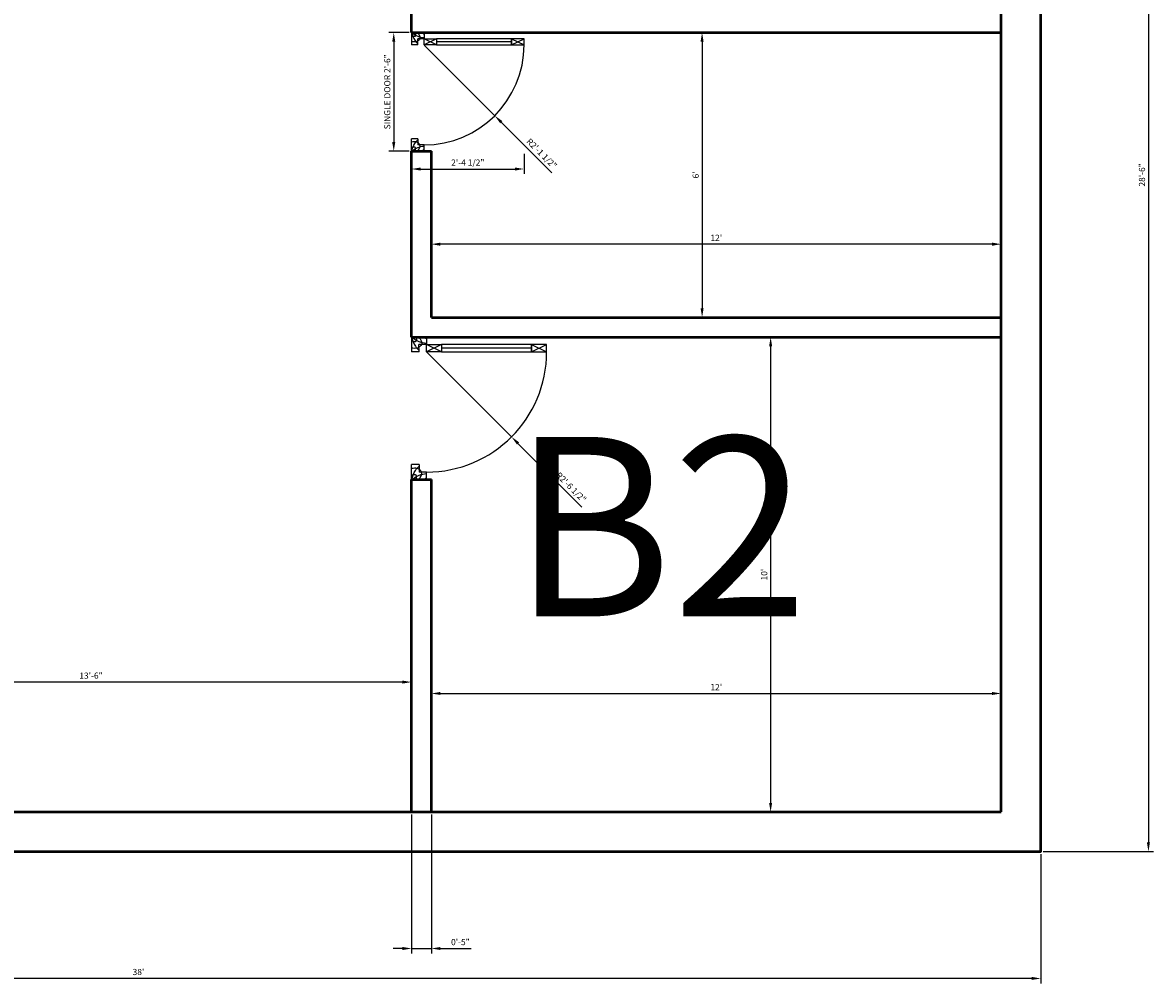
# Model space of a CAD drawing. Units: inches. Extents: x -28 to 484, y -33 to 391.
# Tile 3 of 4: x 199 to 484, y -33 to 209. Entities that reach past the tile are written whole.
import ezdxf

# ---------------------------------------------------------------- set-up
doc = ezdxf.new("R2010")
doc.units = ezdxf.units.IN
for name, color, linetype, lineweight in [('A-ANNO-DIMS', 2, 'Continuous', 18), ('A-AREA-IDEN', 7, 'Continuous', 25), ('A-DOOR', 3, 'Continuous', 25), ('A-WALL', 7, 'Continuous', 50)]:
    doc.layers.add(name, color=color, linetype=linetype, lineweight=lineweight)
doc.styles.get("Standard").update_dxf_attribs({"font": 'arial.ttf'})
doc.dimstyles.new('ISO-25', dxfattribs={"dimtxt": 1.5625, "dimasz": 2.3125, "dimexe": 1.25, "dimexo": 0.625, "dimtad": 1, "dimlunit": 4, "dimtxsty": 'Standard', "dimcen": 2.5, "dimadec": 0, "dimazin": 0, "dimtfac": 1, "dimtmove": 0, "dimatfit": 3, "dimfxl": 1, "dimarcsym": 0})

# ---------------------------------------------------------------- blocks, each defined once
blk = doc.blocks.new('A$C05E21637')
for p, q in [((50, 800), (100, 900)), ((100, 800), (50, 900)), ((75, 800), (75, 200)), ((100, 200), (50, 100)), ((50, 200), (100, 100)), ((0, 100), (0, 0)), ((0, 100), (50, 100)), ((50, 100), (50, 50)), ((900, 100), (900, 50)), ((950, 100), (900, 100)), ((950, 100), (950, 0)), ((100, 50), (50, 50)), ((100, 50), (100, 0)), ((850, 50), (900, 50)), ((850, 50), (850, 0)), ((0, 0), (100, 0)), ((950, 0), (850, 0))]:
    blk.add_line(p, q)
for points in [[(50, 800), (100, 800), (100, 900), (50, 900)], [(50, 200), (100, 200), (100, 800), (50, 800)], [(50, 200), (100, 200), (100, 100), (50, 100)]]:
    blk.add_lwpolyline(points, close=True)
blk.add_arc((100, 100), 800, 0, 90)
for points, knots in [([(0, 0), (11.2, 16), (32.5, 46.3), (38.7, 82.7), (41.2, 100)], [0, 0, 0, 0, 57.729567, 109.527977, 109.527977, 109.527977, 109.527977]), ([(950, 0), (938.8, 16), (917.5, 46.3), (911.3, 82.7), (908.8, 100)], [0, 0, 0, 0, 57.729567, 109.527977, 109.527977, 109.527977, 109.527977]), ([(0, 50), (17.5, 61.3), (46.9, 80.3), (79.6, 38.4), (75.6, 13.1), (73.5, 0)], [0, 0, 0, 0, 52.797078, 89.119952, 128.374378, 128.374378, 128.374378, 128.374378]), ([(0, 0), (21.6, 7.2), (55.2, 18.3), (81.2, 41.3), (90.1, 50)], [0, 0, 0, 0, 67.133415, 104.197904, 104.197904, 104.197904, 104.197904]), ([(0, 30.3), (11.9, 32.6), (36.4, 37.4), (31.4, 12.7), (28.8, 0)], [0, 0, 0, 0, 28.773527, 59.024697, 59.024697, 59.024697, 59.024697]), ([(950, 0), (928.4, 7.2), (894.8, 18.3), (868.8, 41.3), (859.9, 50)], [0, 0, 0, 0, 67.133415, 104.197904, 104.197904, 104.197904, 104.197904]), ([(950, 50), (932.5, 61.3), (903.1, 80.3), (870.4, 38.4), (874.4, 13.1), (876.5, 0)], [0, 0, 0, 0, 52.797078, 89.119952, 128.374378, 128.374378, 128.374378, 128.374378]), ([(950, 30.3), (938.1, 32.6), (913.6, 37.4), (918.6, 12.7), (921.2, 0)], [0, 0, 0, 0, 28.773527, 59.024697, 59.024697, 59.024697, 59.024697])]:
    blk.add_open_spline(points, degree=3, knots=knots)
for points in [[(0, 86.7), (4.7, 91.3), (9.4, 95.9), (15.1, 100)], [(950, 86.7), (945.3, 91.3), (940.6, 95.9), (934.9, 100)]]:
    blk.add_open_spline(points, degree=3)
blk = doc.blocks.new('*D6')
at = {"layer": 'A-ANNO-DIMS', "color": 0, "lineweight": -2, "transparency": 16777216}
for p, q in [((368.18, 207), (371.66, 207)), ((370.41, 204.69), (370.41, 137.31)), ((368.18, 135), (371.66, 135))]:
    blk.add_line(p, q, dxfattribs=at)
at = {"layer": 'A-ANNO-DIMS', "color": 0, "transparency": 16777216}
for points in [[(370.03, 204.69), (370.8, 204.69), (370.41, 207)], [(370.03, 137.31), (370.8, 137.31), (370.41, 135)]]:
    blk.add_solid(points, dxfattribs=at)
at = {"layer": 'Defpoints', "color": 0, "transparency": 16777216}
for p in [(367.55, 207), (367.55, 135), (370.41, 135)]:
    blk.add_point(p, dxfattribs=at)
at = {"layer": 'A-ANNO-DIMS', "color": 0, "transparency": 16777216, "insert": (368.99, 171), "char_height": 1.562, "attachment_point": 5, "rotation": 90}
blk.add_mtext("6'", dxfattribs=at)
blk = doc.blocks.new('*D7')
at = {"layer": 'A-ANNO-DIMS', "color": 0, "lineweight": -2, "transparency": 16777216}
for p, q in [((446, 170.38), (446, 152.25)), ((302, 155.37), (302, 152.25)), ((443.69, 153.5), (304.31, 153.5))]:
    blk.add_line(p, q, dxfattribs=at)
at = {"layer": 'A-ANNO-DIMS', "color": 0, "transparency": 16777216}
for points in [[(304.31, 153.89), (304.31, 153.11), (302, 153.5)], [(443.69, 153.89), (443.69, 153.11), (446, 153.5)]]:
    blk.add_solid(points, dxfattribs=at)
at = {"layer": 'Defpoints', "color": 0, "transparency": 16777216}
for p in [(446, 171), (302, 156), (302, 153.5)]:
    blk.add_point(p, dxfattribs=at)
at = {"layer": 'A-ANNO-DIMS', "color": 0, "transparency": 16777216, "insert": (374, 154.91), "char_height": 1.562, "attachment_point": 5}
blk.add_mtext("12'", dxfattribs=at)
blk = doc.blocks.new('*D8')
at = {"layer": 'A-ANNO-DIMS', "color": 0, "lineweight": -2, "transparency": 16777216}
for p, q in [((388.35, 130), (388.98, 130)), ((387.73, 127.69), (387.73, 12.31)), ((388.35, 10), (388.98, 10))]:
    blk.add_line(p, q, dxfattribs=at)
at = {"layer": 'A-ANNO-DIMS', "color": 0, "transparency": 16777216}
for points in [[(387.34, 127.69), (388.11, 127.69), (387.73, 130)], [(387.34, 12.31), (388.11, 12.31), (387.73, 10)]]:
    blk.add_solid(points, dxfattribs=at)
at = {"layer": 'Defpoints', "color": 0, "transparency": 16777216}
for p in [(387.73, 130), (387.73, 10), (387.73, 10)]:
    blk.add_point(p, dxfattribs=at)
at = {"layer": 'A-ANNO-DIMS', "color": 0, "transparency": 16777216, "insert": (386.31, 70), "char_height": 1.562, "attachment_point": 5, "rotation": 90}
blk.add_mtext("10'", dxfattribs=at)
blk = doc.blocks.new('*D9')
at = {"layer": 'A-ANNO-DIMS', "color": 0, "lineweight": -2, "transparency": 16777216}
for p, q in [((302, 83.23), (302, 38.7)), ((446, 36.98), (446, 41.2)), ((304.31, 39.95), (443.69, 39.95))]:
    blk.add_line(p, q, dxfattribs=at)
at = {"layer": 'A-ANNO-DIMS', "color": 0, "transparency": 16777216}
for points in [[(304.31, 40.34), (304.31, 39.57), (302, 39.95)], [(443.69, 40.34), (443.69, 39.57), (446, 39.95)]]:
    blk.add_solid(points, dxfattribs=at)
at = {"layer": 'Defpoints', "color": 0, "transparency": 16777216}
for p in [(302, 83.85), (446, 39.95), (446, 36.36)]:
    blk.add_point(p, dxfattribs=at)
at = {"layer": 'A-ANNO-DIMS', "color": 0, "transparency": 16777216, "insert": (374, 41.36), "char_height": 1.562, "attachment_point": 5}
blk.add_mtext("12'", dxfattribs=at)
blk = doc.blocks.new('*D10')
at = {"layer": 'A-ANNO-DIMS', "color": 0, "lineweight": -2, "transparency": 16777216}
for p, q in [((135, 51.37), (135, 41.58)), ((297, 51.37), (297, 41.58)), ((294.69, 42.83), (137.31, 42.83))]:
    blk.add_line(p, q, dxfattribs=at)
at = {"layer": 'A-ANNO-DIMS', "color": 0, "transparency": 16777216}
for points in [[(137.31, 43.22), (137.31, 42.45), (135, 42.83)], [(294.69, 43.22), (294.69, 42.45), (297, 42.83)]]:
    blk.add_solid(points, dxfattribs=at)
at = {"layer": 'Defpoints', "color": 0, "transparency": 16777216}
for p in [(135, 52), (297, 52), (135, 42.83)]:
    blk.add_point(p, dxfattribs=at)
at = {"layer": 'A-ANNO-DIMS', "color": 0, "transparency": 16777216, "insert": (216, 44.26), "char_height": 1.562, "attachment_point": 5}
blk.add_mtext('13\'-6"', dxfattribs=at)
blk = doc.blocks.new('*D16')
at = {"layer": 'A-ANNO-DIMS', "color": 0, "lineweight": -2, "transparency": 16777216}
for p, q in [((456.63, 342), (484.44, 342)), ((483.19, 339.69), (483.19, 2.31)), ((456.63, 0), (484.44, 0))]:
    blk.add_line(p, q, dxfattribs=at)
at = {"layer": 'A-ANNO-DIMS', "color": 0, "transparency": 16777216}
for points in [[(482.8, 339.69), (483.57, 339.69), (483.19, 342)], [(482.8, 2.31), (483.57, 2.31), (483.19, 0)]]:
    blk.add_solid(points, dxfattribs=at)
at = {"layer": 'Defpoints', "color": 0, "transparency": 16777216}
for p in [(456, 342), (456, 0), (483.19, 0)]:
    blk.add_point(p, dxfattribs=at)
at = {"layer": 'A-ANNO-DIMS', "color": 0, "transparency": 16777216, "insert": (481.76, 171), "char_height": 1.562, "attachment_point": 5, "rotation": 90}
blk.add_mtext('28\'-6"', dxfattribs=at)
blk = doc.blocks.new('*D18')
at = {"layer": 'A-ANNO-DIMS', "color": 0, "lineweight": -2, "transparency": 16777216}
for p, q in [((0, -0.62), (0, -33.32)), ((456, -0.62), (456, -33.32)), ((453.69, -32.07), (2.31, -32.07))]:
    blk.add_line(p, q, dxfattribs=at)
at = {"layer": 'A-ANNO-DIMS', "color": 0, "transparency": 16777216}
for points in [[(2.31, -31.68), (2.31, -32.45), (0, -32.07)], [(453.69, -31.68), (453.69, -32.45), (456, -32.07)]]:
    blk.add_solid(points, dxfattribs=at)
at = {"layer": 'Defpoints', "color": 0, "transparency": 16777216}
for p in [(0, 0), (456, 0), (0, -32.07)]:
    blk.add_point(p, dxfattribs=at)
at = {"layer": 'A-ANNO-DIMS', "color": 0, "transparency": 16777216, "insert": (228, -30.64), "char_height": 1.562, "attachment_point": 5}
blk.add_mtext("38'", dxfattribs=at)
blk = doc.blocks.new('*D22')
at = {"layer": 'A-ANNO-DIMS', "color": 0, "lineweight": -2, "transparency": 16777216}
for p, q in [((296.37, 207), (291.25, 207)), ((292.5, 204.69), (292.5, 179.31)), ((296.37, 177), (291.25, 177))]:
    blk.add_line(p, q, dxfattribs=at)
at = {"layer": 'A-ANNO-DIMS', "color": 0, "transparency": 16777216}
for points in [[(292.11, 204.69), (292.89, 204.69), (292.5, 207)], [(292.11, 179.31), (292.89, 179.31), (292.5, 177)]]:
    blk.add_solid(points, dxfattribs=at)
at = {"layer": 'Defpoints', "color": 0, "transparency": 16777216}
for p in [(297, 207), (292.5, 177), (297, 177)]:
    blk.add_point(p, dxfattribs=at)
at = {"layer": 'A-ANNO-DIMS', "color": 0, "transparency": 16777216, "insert": (291.07, 192), "char_height": 1.5625, "attachment_point": 5, "rotation": 90}
blk.add_mtext('SINGLE DOOR 2\'-6"', dxfattribs=at)
blk = doc.blocks.new('*D23')
at = {"layer": 'A-ANNO-DIMS', "color": 0, "lineweight": -2, "transparency": 16777216}
for p, q in [((297, 176.37), (297, 171.25)), ((325.42, 176.37), (325.42, 171.25)), ((299.31, 172.5), (323.11, 172.5))]:
    blk.add_line(p, q, dxfattribs=at)
at = {"layer": 'A-ANNO-DIMS', "color": 0, "transparency": 16777216}
for points in [[(299.31, 172.89), (299.31, 172.11), (297, 172.5)], [(323.11, 172.89), (323.11, 172.11), (325.42, 172.5)]]:
    blk.add_solid(points, dxfattribs=at)
at = {"layer": 'Defpoints', "color": 0, "transparency": 16777216}
for p in [(297, 177), (325.42, 177), (325.42, 172.5)]:
    blk.add_point(p, dxfattribs=at)
at = {"layer": 'A-ANNO-DIMS', "color": 0, "transparency": 16777216, "insert": (311.21, 173.93), "char_height": 1.562, "attachment_point": 5}
blk.add_mtext('2\'-4 1/2"', dxfattribs=at)
blk = doc.blocks.new('*D38')
at = {"layer": 'A-ANNO-DIMS', "color": 0, "lineweight": -2, "transparency": 16777216}
for p, q in [((297, 9.38), (297, -25.75)), ((302, 9.38), (302, -25.75)), ((294.69, -24.5), (292.38, -24.5)), ((297, -24.5), (302, -24.5)), ((304.31, -24.5), (312.03, -24.5))]:
    blk.add_line(p, q, dxfattribs=at)
at = {"layer": 'A-ANNO-DIMS', "color": 0, "transparency": 16777216}
for points in [[(294.69, -24.11), (294.69, -24.89), (297, -24.5)], [(304.31, -24.11), (304.31, -24.89), (302, -24.5)]]:
    blk.add_solid(points, dxfattribs=at)
at = {"layer": 'Defpoints', "color": 0, "transparency": 16777216}
for p in [(297, 10), (302, 10), (302, -24.5)]:
    blk.add_point(p, dxfattribs=at)
at = {"layer": 'A-ANNO-DIMS', "color": 0, "transparency": 16777216, "insert": (309.33, -23.08), "char_height": 1.562, "attachment_point": 5}
blk.add_mtext('0\'-5"', dxfattribs=at)
blk = doc.blocks.new('*D40')
at = {"layer": 'A-ANNO-DIMS', "color": 0, "lineweight": -2, "transparency": 16777216}
for p, q in [((300.78, 126.26), (322.26, 104.8)), ((340.06, 87.02), (323.89, 103.17))]:
    blk.add_line(p, q, dxfattribs=at)
at = {"layer": 'A-ANNO-DIMS', "color": 0, "transparency": 16777216}
blk.add_solid([(324.17, 103.44), (323.62, 102.89), (322.26, 104.8)], dxfattribs=at)
at = {"layer": 'Defpoints', "color": 0, "transparency": 16777216}
for p in [(300.78, 126.26), (322.26, 104.8)]:
    blk.add_point(p, dxfattribs=at)
at = {"layer": 'A-ANNO-DIMS', "color": 0, "transparency": 16777216, "insert": (336.16, 92.94), "char_height": 1.5625, "attachment_point": 5, "rotation": 315.0277}
blk.add_mtext('3X R2\'-6 1/2"', dxfattribs=at)
blk = doc.blocks.new('*D43')
at = {"layer": 'A-ANNO-DIMS', "color": 0, "lineweight": -2, "transparency": 16777216}
for p, q in [((300.16, 203.84), (318.02, 185.98)), ((332.47, 171.53), (319.66, 184.34))]:
    blk.add_line(p, q, dxfattribs=at)
at = {"layer": 'A-ANNO-DIMS', "color": 0, "transparency": 16777216}
blk.add_solid([(319.93, 184.62), (319.38, 184.07), (318.02, 185.98)], dxfattribs=at)
at = {"layer": 'Defpoints', "color": 0, "transparency": 16777216}
for p in [(300.16, 203.84), (318.02, 185.98)]:
    blk.add_point(p, dxfattribs=at)
at = {"layer": 'A-ANNO-DIMS', "color": 0, "transparency": 16777216, "insert": (329.75, 176.27), "char_height": 1.562, "attachment_point": 5, "rotation": 315}
blk.add_mtext('R2\'-1 1/2"', dxfattribs=at)

msp = doc.modelspace()

# ---------------------------------------------------------------- linework, layer by layer
at = {"layer": 'A-WALL'}
for p, q in [((446, 10), (446, 332)), ((297, 207), (297, 212)), ((297, 207), (446, 207)), ((297, 177), (302, 177)), ((297, 130), (297, 177)), ((302, 135), (302, 177)), ((302, 135), (446, 135)), ((297, 130), (446, 130)), ((297, 10), (297, 94)), ((297, 94), (302, 94)), ((302, 10), (302, 94)), ((10, 10), (446, 10))]:
    msp.add_line(p, q, dxfattribs=at)
msp.add_lwpolyline([(0, 258), (0, 0), (456, 0), (456, 342), (0, 342)], dxfattribs=at)

# ---------------------------------------------------------------- block references
at = {"layer": 'A-DOOR'}
for p, xscale, yscale, zscale, rotation in [((297, 207), 0.0315789473684211, 0.0315789473684211, 0.0315789473684211, 269.9999999999992), ((296.983, 130.052), 0.0379493754661746, 0.0379493754661746, 0.0379493754661746, 270.0274398095227)]:
    msp.add_blockref('A$C05E21637', p, dxfattribs=dict(at, xscale=xscale, yscale=yscale, zscale=zscale, rotation=rotation))

# ---------------------------------------------------------------- texts
at = {"layer": 'A-AREA-IDEN', "insert": (322.257, 104.802), "char_height": 45.3593, "attachment_point": 1}
msp.add_mtext_dynamic_manual_height_columns('B2', width=51.74282, gutter_width=226.796, heights=[0], dxfattribs=at)

# ---------------------------------------------------------------- dimensions: what is measured, and where the dimension line sits
at = {"layer": 'A-ANNO-DIMS'}
for base, p1, p2, picture, middle in [((483.187, 0), (456, 342), (456, 0), '*D16', (481.765, 171)), ((370.411, 135), (367.551, 207), (367.551, 135), '*D6', (368.988, 171)), ((387.728, 10), (387.728, 130), (387.728, 10), '*D8', (386.306, 70))]:
    dim = msp.add_linear_dim(base=base, p1=p1, p2=p2, angle=90, dimstyle='ISO-25', override={"dimclrd": 0, "dimclre": 0, "dimclrt": 0}, dxfattribs=at)
    dim.commit()
    dim.dimension.update_dxf_attribs({"geometry": picture, "text_midpoint": middle})
dim = msp.add_linear_dim(base=(292.5, 177), p1=(297, 207), p2=(297, 177), angle=270, text='SINGLE DOOR <>', dimstyle='ISO-25', override={"dimdec": 1, "dimlfac": 1, "dimrnd": 0, "dimzin": 1, "dimdsep": 46, "dimlunit": 4, "dimfrac": 2}, dxfattribs=at)
dim.commit()
dim.dimension.update_dxf_attribs({"geometry": '*D22', "text_midpoint": (291.067, 192)})
dim = msp.add_radius_dim(center=(300.158, 203.842), mpoint=(318.022, 185.978), dimstyle='ISO-25', override={"dimdec": 1, "dimlfac": 1, "dimrnd": 0, "dimzin": 1, "dimdsep": 46, "dimlunit": 4, "dimfrac": 2}, dxfattribs=at)
dim.commit()
dim.dimension.update_dxf_attribs({"geometry": '*D43', "text_midpoint": (328.74, 175.26), "dimtype": 164})
for base, p1, p2, override, picture, middle in [((325.421, 172.5), (297, 177), (325.421, 177), {"dimdec": 1, "dimlfac": 1, "dimrnd": 0, "dimzin": 1, "dimdsep": 46, "dimlunit": 4, "dimfrac": 2}, '*D23', (311.211, 173.933)), ((302, 153.5), (446, 171), (302, 156), {"dimclrd": 0, "dimclre": 0, "dimclrt": 0}, '*D7', (374, 154.909)), ((446, 39.955), (302, 83.851), (446, 36.357), {"dimclrd": 0, "dimclre": 0, "dimclrt": 0}, '*D9', (374, 41.364)), ((135, 42.833), (297, 52), (135, 52), {"dimclrd": 0, "dimclre": 0, "dimclrt": 0}, '*D10', (216, 44.257)), ((302, -24.5), (297, 10), (302, 10), {"dimdec": 1, "dimlfac": 1, "dimrnd": 0, "dimzin": 1, "dimdsep": 46, "dimlunit": 4, "dimfrac": 2}, '*D38', (309.327, -23.077)), ((0, -32.067), (456, 0), (0, 0), {"dimclrd": 0, "dimclre": 0, "dimclrt": 0}, '*D18', (228, -30.644))]:
    dim = msp.add_linear_dim(base=base, p1=p1, p2=p2, dimstyle='ISO-25', override=override, dxfattribs=at)
    dim.commit()
    dim.dimension.update_dxf_attribs({"geometry": picture, "text_midpoint": middle})
dim = msp.add_radius_dim(center=(300.779, 126.259), mpoint=(322.257, 104.802), text='3X <>', dimstyle='ISO-25', override={"dimdec": 1, "dimlfac": 1, "dimrnd": 0, "dimzin": 1, "dimdsep": 46, "dimlunit": 4, "dimfrac": 2}, dxfattribs=at)
dim.commit()
dim.dimension.update_dxf_attribs({"geometry": '*D40', "text_midpoint": (335.144, 91.928), "dimtype": 164})

doc.saveas('drawing.dxf')
